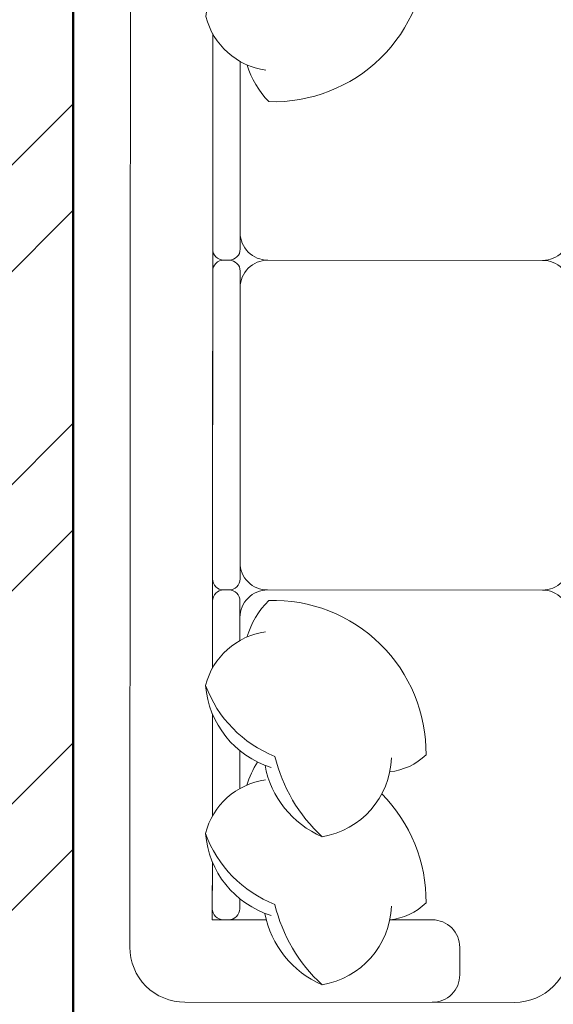
# Model space of a CAD drawing. Units: inches. Extents: x 963 to 2075, y 289 to 2657.
# Tile 83 of 98: x 1511 to 1533, y 2243 to 2284. Entities that reach past the tile are written whole.
import ezdxf

# ---------------------------------------------------------------- set-up
doc = ezdxf.new("R2010")
doc.units = ezdxf.units.IN
for name, color, linetype, lineweight in [('A-FURN', 8, 'Continuous', 18), ('A-WALL', 7, 'Continuous', 50), ('A-WALL-PATT', 8, 'Continuous', 13)]:
    doc.layers.add(name, color=color, linetype=linetype, lineweight=lineweight)

# ---------------------------------------------------------------- blocks, each defined once
blk = doc.blocks.new('SOFA-3SEAT')
at = {"ltscale": 0.03}
blk.add_lwpolyline([(2.442, 16.426, -0.414214), (0.124, 18.743), (0.124, 32.649, -0.414214), (1.283, 33.808, -0.414214), (0.124, 34.967), (0.124, 46.555, -0.414214), (1.283, 47.713, -0.414214), (0.124, 48.872), (0.124, 62.778, -0.414214), (2.442, 65.095), (16.347, 65.095, -0.414214), (18.665, 62.778), (18.665, 18.743, -0.414214), (16.347, 16.426)], format="xyb", close=True, dxfattribs=at)
for points in [[(7.713, 61.619), (5.918, 61.619, -0.414214), (4.759, 62.778), (4.759, 63.937, -0.414214), (5.918, 65.095)], [(7.643, 61.038, -0.356772), (10.564, 64.358, -0.249542), (12.971, 61.349, 9.61688)], [(10.564, 64.358, -0.14773), (12.556, 60.971, -0.213343), (15.477, 57.983, -0.178662)], [(7.714, 61.622, 0.165541), (6.183, 60.905, 0.200231), (8.048, 56.305, 0.121523)], [(15.189, 59.181), (15.189, 61.619), (12.911, 61.619, -0.414214)], [(14.03, 60.735), (14.03, 61.156, -0.414214), (14.493, 61.619), (14.725, 61.619, -0.414214), (15.189, 61.156)], [(12.714, 61.439, -0.306663), (15.477, 57.983, -0.30633), (12.954, 55.725, 0.872847)], [(15.189, 61.156), (15.189, 59.181, -0.414214)], [(7.643, 54.795, -0.356772), (10.564, 58.116, -0.249542), (12.971, 55.107, 9.61688)], [(10.564, 58.116, -0.14773), (12.556, 54.729, -0.213343), (15.477, 51.74, -0.178662)], [(15.189, 57.253), (15.189, 52.939, -0.414214)], [(14.03, 54.492), (14.03, 56.087, -0.414214)], [(13.283, 54.97, 0.071865), (13.736, 55.942, -7.115464)], [(7.714, 55.379, 0.165541), (6.183, 54.662, 0.425989), (12.821, 48.154, 0.121523), (13.736, 49.699, -7.115464)], [(12.714, 55.197, -0.306663), (15.477, 51.74, -0.30633), (12.954, 49.482, 0.872847)], [(15.189, 51.011), (15.189, 48.177, -0.414214), (14.725, 47.713), (14.493, 47.713, -0.414214), (14.03, 48.177), (14.03, 49.844, -0.414214)], [(14.03, 48.872, -0.414214), (12.871, 47.713), (1.283, 47.713, -0.414214)], [(14.03, 46.555, 0.414214), (12.871, 47.713)], [(14.03, 34.967, -0.414214), (12.871, 33.808)], [(14.03, 32.649, 0.414214), (12.871, 33.808), (1.283, 33.808, 0.414214)], [(15.189, 24.268), (15.189, 33.344, 0.414214), (14.725, 33.808), (14.493, 33.808, 0.414214), (14.03, 33.344), (14.03, 25.435, 0.414214)], [(7.714, 19.9, -0.165541), (6.183, 20.616, -0.425989), (12.821, 27.124, -0.121523), (13.736, 25.58, 7.115464)], [(12.714, 20.082, 0.306663), (15.477, 23.538, 0.30633), (12.954, 25.796, -0.872847)]]:
    blk.add_lwpolyline(points, format="xyb")
for points in [[(15.189, 52.939), (15.189, 57.253)], [(15.189, 24.268), (15.189, 51.011)]]:
    blk.add_lwpolyline(points)
blk.add_lwpolyline([(15.189, 47.25), (15.189, 34.271, -0.414214), (14.725, 33.808), (14.493, 33.808, -0.414214), (14.03, 34.271), (14.03, 47.25, -0.414214), (14.493, 47.713), (14.725, 47.713, -0.414214)], format="xyb", close=True)

msp = doc.modelspace()

# ---------------------------------------------------------------- hatches: boundary and pattern name
at = {"layer": 'A-WALL-PATT'}
h = msp.add_hatch(dxfattribs=at)
h.set_pattern_fill('ANSI32', color=256)
h.paths.add_polyline_path([(1296.922, 2558.318), (1203.922, 2558.318), (1203.922, 2493.818), (1191.533, 2493.818), (1191.533, 2489.318), (1211.063, 2489.318), (1211.063, 2492.02), (1211.063, 2493.818), (1208.422, 2493.818), (1208.422, 2553.818), (1292.422, 2553.818), (1292.422, 2538.863), (1296.922, 2538.863)])
h.paths.add_polyline_path([(1442.422, 2558.318), (1349.422, 2558.318), (1349.422, 2538.943), (1353.922, 2538.943), (1353.922, 2553.818), (1437.922, 2553.818), (1437.922, 2493.818), (1434.542, 2493.818), (1434.542, 2489.318), (1448.311, 2489.318), (1448.311, 2491.568), (1448.311, 2493.818), (1442.422, 2493.818)])
h.paths.add_polyline_path([(1415.554, 2491.568), (1415.554, 2493.818), (1340.941, 2493.818), (1340.941, 2489.318), (1371.922, 2489.318), (1371.922, 2378.318), (1367.596, 2378.318), (1367.596, 2373.818), (1371.922, 2373.818), (1371.922, 2355.185), (1376.422, 2355.185), (1376.422, 2489.318), (1415.554, 2489.318)])
h.paths.add_polyline_path([(1304.941, 2491.568), (1304.941, 2493.818), (1296.922, 2493.818), (1296.922, 2514.863), (1292.422, 2514.863), (1292.422, 2493.818), (1232.808, 2493.818), (1232.808, 2489.318), (1256.422, 2489.318), (1256.422, 2327.318), (1253.714, 2327.318), (1253.714, 2322.818), (1328.422, 2322.818), (1328.422, 2331.147), (1323.922, 2331.147), (1323.922, 2327.318), (1260.922, 2327.318), (1260.922, 2373.818), (1323.922, 2373.818), (1323.922, 2357.812), (1328.422, 2357.812), (1328.422, 2373.818), (1346.007, 2373.818), (1346.007, 2376.068), (1346.007, 2378.318), (1260.922, 2378.318), (1260.922, 2489.318), (1304.941, 2489.318)])
h.paths.add_polyline_path([(1226.654, 2327.318), (1124.422, 2327.318), (1124.422, 2347.447), (1119.922, 2347.447), (1119.922, 2322.818), (1163.422, 2322.818), (1163.422, 2305.435), (1165.672, 2305.435), (1167.922, 2305.435), (1167.922, 2322.818), (1226.654, 2322.818), (1226.654, 2325.068)])
h.paths.add_polyline_path([(1095.922, 2489.318), (1124.422, 2489.318), (1131.533, 2489.318), (1131.533, 2491.568), (1131.533, 2493.818), (1119.922, 2493.818), (1091.422, 2493.818), (1091.422, 2417.318), (1095.922, 2417.318), (1119.922, 2417.318), (1119.922, 2407.447), (1124.422, 2407.447), (1124.422, 2421.818), (1095.922, 2421.818)])
h.paths.add_polyline_path([(1512.922, 2558.318), (1508.422, 2558.318), (1508.422, 2493.818), (1503.401, 2493.818), (1503.401, 2489.318), (1508.422, 2489.318), (1508.422, 2327.318), (1376.422, 2327.318), (1376.422, 2330.273), (1371.922, 2330.273), (1371.922, 2298.744), (1376.422, 2298.744), (1376.422, 2322.818), (1508.422, 2322.818), (1508.422, 2165.318), (1504.255, 2165.318), (1504.255, 2160.818), (1508.422, 2160.818), (1508.422, 2108.318), (1512.922, 2108.318), (1512.922, 2160.818), (1516.182, 2160.818), (1516.182, 2163.068), (1516.182, 2165.318), (1512.922, 2165.318), (1512.922, 2322.818), (1644.922, 2322.818), (1644.922, 2298.744), (1649.422, 2298.744), (1649.422, 2322.818), (1649.422, 2330.944), (1647.172, 2330.944), (1644.922, 2330.944), (1644.922, 2327.318), (1512.922, 2327.318), (1512.922, 2489.318), (1516.759, 2489.318), (1516.759, 2491.568), (1516.759, 2493.818), (1512.922, 2493.818)])
h.paths.add_polyline_path([(1671.922, 2558.318), (1578.922, 2558.318), (1578.922, 2493.818), (1573.526, 2493.818), (1573.526, 2489.318), (1586.537, 2489.318), (1586.537, 2491.568), (1586.537, 2493.818), (1583.422, 2493.818), (1583.422, 2553.818), (1667.422, 2553.818), (1667.422, 2541.109), (1671.922, 2541.109)])
h.paths.add_polyline_path([(1681.257, 2493.818), (1671.922, 2493.818), (1671.922, 2517.109), (1667.422, 2517.109), (1667.422, 2493.818), (1610.218, 2493.818), (1610.218, 2489.318), (1644.922, 2489.318), (1644.922, 2357.865), (1649.422, 2357.865), (1649.422, 2373.818), (1652.203, 2373.818), (1652.203, 2375.827), (1652.203, 2378.318), (1649.422, 2378.318), (1649.422, 2489.318), (1681.257, 2489.318), (1681.257, 2491.568)])
h.paths.add_polyline_path([(1821.922, 2558.318), (1728.922, 2558.318), (1728.922, 2541), (1733.422, 2541), (1733.422, 2553.818), (1817.422, 2553.818), (1817.422, 2493.818), (1813.507, 2493.818), (1813.507, 2489.318), (1830.078, 2489.318), (1830.078, 2491.568), (1830.078, 2493.818), (1821.922, 2493.818)])
h.paths.add_polyline_path([(1794.244, 2493.818), (1717.257, 2493.818), (1717.257, 2489.318), (1760.422, 2489.318), (1760.422, 2378.318), (1674.401, 2378.318), (1674.401, 2373.818), (1692.922, 2373.818), (1692.922, 2356.954), (1697.422, 2356.954), (1697.422, 2373.818), (1760.422, 2373.818), (1760.422, 2327.318), (1697.422, 2327.318), (1697.422, 2333.341), (1692.922, 2333.341), (1692.922, 2322.818), (1768.037, 2322.818), (1768.037, 2325.068), (1768.037, 2327.318), (1764.922, 2327.318), (1764.922, 2489.318), (1794.244, 2489.318)])
h.paths.add_polyline_path([(1733.422, 2517), (1728.922, 2517), (1728.922, 2493.818), (1733.422, 2493.818)], flags=17)
h.paths.add_polyline_path([(1929.922, 2493.818), (1890.078, 2493.818), (1890.078, 2489.318), (1896.922, 2489.318), (1925.422, 2489.318), (1925.422, 2421.818), (1896.922, 2421.818), (1896.922, 2408.318), (1901.422, 2408.318), (1901.422, 2417.318), (1925.422, 2417.318), (1929.922, 2417.318)])
h.paths.add_polyline_path([(1901.422, 2348.318), (1896.922, 2348.318), (1896.922, 2327.318), (1800.423, 2327.318), (1800.423, 2322.818), (1853.422, 2322.818), (1853.422, 2309.453), (1857.922, 2309.453), (1857.922, 2322.818), (1901.422, 2322.818)])
h.paths.add_polyline_path([(1857.922, 2249.453), (1853.422, 2249.453), (1853.422, 2214.818), (1686.309, 2214.818), (1686.309, 2210.318), (1853.422, 2210.318), (1853.422, 2202.134), (1857.922, 2202.134), (1857.922, 2210.318)])
h.paths.add_polyline_path([(1857.922, 2142.134), (1853.422, 2142.134), (1853.422, 2115.422), (1841.422, 2115.422), (1841.422, 2088.531), (1841.422, 2046.949), (1845.922, 2046.949), (1845.922, 2110.922), (1905.922, 2110.922), (1905.922, 2092.517), (1910.422, 2092.517), (1910.422, 2115.422), (1857.922, 2115.422)])
h.paths.add_polyline_path([(1532.436, 1482.342), (1573.456, 1482.342), (1573.456, 1501), (1532.436, 1501)], flags=9)
h.paths.add_polyline_path([(1438.658, 1486.302), (1479.678, 1486.302), (1479.678, 1504.96), (1438.658, 1504.96)], flags=9)
h.paths.add_polyline_path([(1411.215, 1365.308), (1659.139, 1365.308), (1659.139, 1402.401), (1411.215, 1402.401)], flags=9)
h.paths.add_polyline_path([(1185.671, 2296.298), (1248.16, 2296.298), (1248.16, 2314.955), (1185.671, 2314.955)], flags=9)
h.paths.add_polyline_path([(1177.31, 2187.35), (1216.15, 2187.35), (1216.15, 2206.007), (1177.31, 2206.007)], flags=9)
h.paths.add_polyline_path([(1295.101, 1602.083), (1328.26, 1602.083), (1328.26, 1620.741), (1295.101, 1620.741)], flags=9)
h.paths.add_polyline_path([(1525.126, 2005.99), (1558.39, 2005.99), (1558.39, 2024.648), (1525.126, 2024.648)], flags=9)
h.paths.add_polyline_path([(1459.606, 1977.125), (1472.195, 1977.125), (1472.195, 1987.429), (1459.606, 1987.429)], flags=9)
h.paths.add_polyline_path([(1467.815, 2053.676), (1480.018, 2053.676), (1480.018, 2063.979), (1467.815, 2063.979)], flags=9)
h.paths.add_polyline_path([(1555.184, 2119.02), (1584.563, 2119.02), (1584.563, 2137.678), (1555.184, 2137.678)], flags=25)
h.paths.add_polyline_path([(1405.389, 2115.291), (1444.478, 2115.291), (1444.478, 2133.948), (1405.389, 2133.948)], flags=25)
h.paths.add_polyline_path([(1698.482, 2004.259), (1727.695, 2004.259), (1727.695, 2022.916), (1698.482, 2022.916)], flags=9)
h.paths.add_polyline_path([(1612.158, 1972.855), (1629.016, 1972.855), (1629.016, 1983.159), (1612.158, 1983.159)], flags=9)
h.paths.add_polyline_path([(1608.289, 2060.036), (1625.147, 2060.036), (1625.147, 2070.34), (1608.289, 2070.34)], flags=9)
h.paths.add_polyline_path([(1527.954, 1684.402), (1566.795, 1684.402), (1566.795, 1703.06), (1527.954, 1703.06)], flags=9)
h.paths.add_polyline_path([(1422.792, 1683.59), (1461.633, 1683.59), (1461.633, 1702.247), (1422.792, 1702.247)], flags=9)
h.paths.add_polyline_path([(1531.262, 1732.459), (1574.015, 1732.459), (1574.015, 1751.116), (1531.262, 1751.116)], flags=9)
h.paths.add_polyline_path([(1402.872, 1732.845), (1439.799, 1732.845), (1439.799, 1751.502), (1402.872, 1751.502)], flags=9)
h.paths.add_polyline_path([(1243.122, 1923.132), (1281.962, 1923.132), (1281.962, 1941.79), (1243.122, 1941.79)], flags=9)
h.paths.add_polyline_path([(1181.752, 1792.268), (1244.241, 1792.268), (1244.241, 1810.926), (1181.752, 1810.926)], flags=9)
h.paths.add_polyline_path([(1265.822, 1670.3), (1316.071, 1670.3), (1316.071, 1688.957), (1265.822, 1688.957)], flags=9)
h.paths.add_polyline_path([(1140.263, 1676.054), (1179.104, 1676.054), (1179.104, 1694.711), (1140.263, 1694.711)], flags=9)
h.paths.add_polyline_path([(1107.49, 1490.889), (1143.374, 1490.889), (1143.374, 1509.546), (1107.49, 1509.546)], flags=9)
h.paths.add_polyline_path([(1217.584, 1483.899), (1246.741, 1483.899), (1246.741, 1502.556), (1217.584, 1502.556)], flags=9)
h.paths.add_polyline_path([(1389.21, 1486.919), (1418.367, 1486.919), (1418.367, 1505.576), (1389.21, 1505.576)], flags=9)
h.paths.add_polyline_path([(1672.208, 1602.083), (1705.366, 1602.083), (1705.366, 1620.741), (1672.208, 1620.741)], flags=9)
h.paths.add_polyline_path([(1752.082, 1522.638), (1781.24, 1522.638), (1781.24, 1541.295), (1752.082, 1541.295)], flags=9)
h.paths.add_polyline_path([(1848.275, 1491.26), (1884.158, 1491.26), (1884.158, 1509.918), (1848.275, 1509.918)], flags=9)
h.paths.add_polyline_path([(1822.47, 1685.62), (1861.31, 1685.62), (1861.31, 1704.278), (1822.47, 1704.278)], flags=9)
h.paths.add_polyline_path([(1713.195, 1672.232), (1763.444, 1672.232), (1763.444, 1690.889), (1713.195, 1690.889)], flags=9)
h.paths.add_polyline_path([(1736.619, 1790.578), (1799.109, 1790.578), (1799.109, 1809.235), (1736.619, 1809.235)], flags=9)
h.paths.add_polyline_path([(1691.491, 1916.355), (1730.332, 1916.355), (1730.332, 1935.013), (1691.491, 1935.013)], flags=9)
h.paths.add_polyline_path([(1764.872, 1973.922), (1794.306, 1973.922), (1794.306, 1992.58), (1764.872, 1992.58)], flags=9)
h.paths.add_polyline_path([(1767.854, 2034.017), (1797.288, 2034.017), (1797.288, 2052.674), (1767.854, 2052.674)], flags=9)
h.paths.add_polyline_path([(1851.593, 2060.331), (1880.751, 2060.331), (1880.751, 2078.989), (1851.593, 2078.989)], flags=25)
h.paths.add_polyline_path([(1688.491, 2086.874), (1727.332, 2086.874), (1727.332, 2105.531), (1688.491, 2105.531)], flags=9)
h.paths.add_polyline_path([(1537.743, 2293.581), (1580.495, 2293.581), (1580.495, 2312.239), (1537.743, 2312.239)], flags=25)
h.paths.add_polyline_path([(1425.587, 2296.109), (1468.34, 2296.109), (1468.34, 2314.766), (1425.587, 2314.766)], flags=25)
h.paths.add_polyline_path([(1278.518, 2004.184), (1307.72, 2004.184), (1307.72, 2022.841), (1278.518, 2022.841)], flags=9)
h.paths.add_polyline_path([(1193.282, 1973.635), (1222.715, 1973.635), (1222.715, 1992.292), (1193.282, 1992.292)], flags=9)
h.paths.add_polyline_path([(1192.411, 2040.577), (1221.845, 2040.577), (1221.845, 2059.234), (1192.411, 2059.234)], flags=9)
h.paths.add_polyline_path([(1130.603, 1951.393), (1159.76, 1951.393), (1159.76, 1970.05), (1130.603, 1970.05)], flags=9)
h.paths.add_polyline_path([(1132.827, 2052.494), (1161.984, 2052.494), (1161.984, 2071.151), (1132.827, 2071.151)], flags=9)
h.paths.add_polyline_path([(1265.128, 2334.619), (1315.377, 2334.619), (1315.377, 2353.277), (1265.128, 2353.277)], flags=25)
h.paths.add_polyline_path([(1136.741, 2330.785), (1175.582, 2330.785), (1175.582, 2349.443), (1136.741, 2349.443)], flags=9)
h.paths.add_polyline_path([(1287.422, 2417.204), (1320.58, 2417.204), (1320.58, 2435.861), (1287.422, 2435.861)], flags=25)
h.paths.add_polyline_path([(1430.988, 2329.159), (1469.828, 2329.159), (1469.828, 2347.816), (1430.988, 2347.816)], flags=25)
h.paths.add_polyline_path([(1525.424, 2329.213), (1564.264, 2329.213), (1564.264, 2347.87), (1525.424, 2347.87)], flags=25)
h.paths.add_polyline_path([(1684.525, 2382.799), (1717.683, 2382.799), (1717.683, 2401.457), (1684.525, 2401.457)], flags=25)
h.paths.add_polyline_path([(1704.805, 2340.293), (1755.054, 2340.293), (1755.054, 2358.95), (1704.805, 2358.95)], flags=25)
h.paths.add_polyline_path([(1694.113, 2287.757), (1756.602, 2287.757), (1756.602, 2306.414), (1694.113, 2306.414)], flags=9)
h.paths.add_polyline_path([(1815.778, 2329.861), (1854.618, 2329.861), (1854.618, 2348.518), (1815.778, 2348.518)], flags=9)
h.paths.add_polyline_path([(1842.873, 2514.256), (1878.756, 2514.256), (1878.756, 2532.914), (1842.873, 2532.914)], flags=9)
h.paths.add_polyline_path([(1769.513, 2531.447), (1798.671, 2531.447), (1798.671, 2550.104), (1769.513, 2550.104)], flags=25)
h.paths.add_polyline_path([(1594.772, 2518.468), (1623.93, 2518.468), (1623.93, 2537.125), (1594.772, 2537.125)], flags=25)
h.paths.add_polyline_path([(1520.723, 2516.185), (1556.606, 2516.185), (1556.606, 2534.842), (1520.723, 2534.842)], flags=25)
h.paths.add_polyline_path([(1464.456, 2516.694), (1500.34, 2516.694), (1500.34, 2535.351), (1464.456, 2535.351)], flags=25)
h.paths.add_polyline_path([(1365.696, 2528.97), (1394.854, 2528.97), (1394.854, 2547.627), (1365.696, 2547.627)], flags=25)
h.paths.add_polyline_path([(1222.838, 2516.231), (1251.995, 2516.231), (1251.995, 2534.889), (1222.838, 2534.889)], flags=25)
h.paths.add_polyline_path([(1104.545, 2509.6), (1140.429, 2509.6), (1140.429, 2528.257), (1104.545, 2528.257)], flags=9)

# ---------------------------------------------------------------- linework, layer by layer
at = {"layer": 'A-WALL'}
msp.add_line((1512.922, 2165.318), (1512.922, 2322.818), dxfattribs=at)

# ---------------------------------------------------------------- block references
at = {"layer": 'A-FURN', "rotation": 179.9690487318625}
msp.add_blockref('SOFA-3SEAT', (1534.012, 2307.942), dxfattribs=at)

doc.saveas('drawing.dxf')
